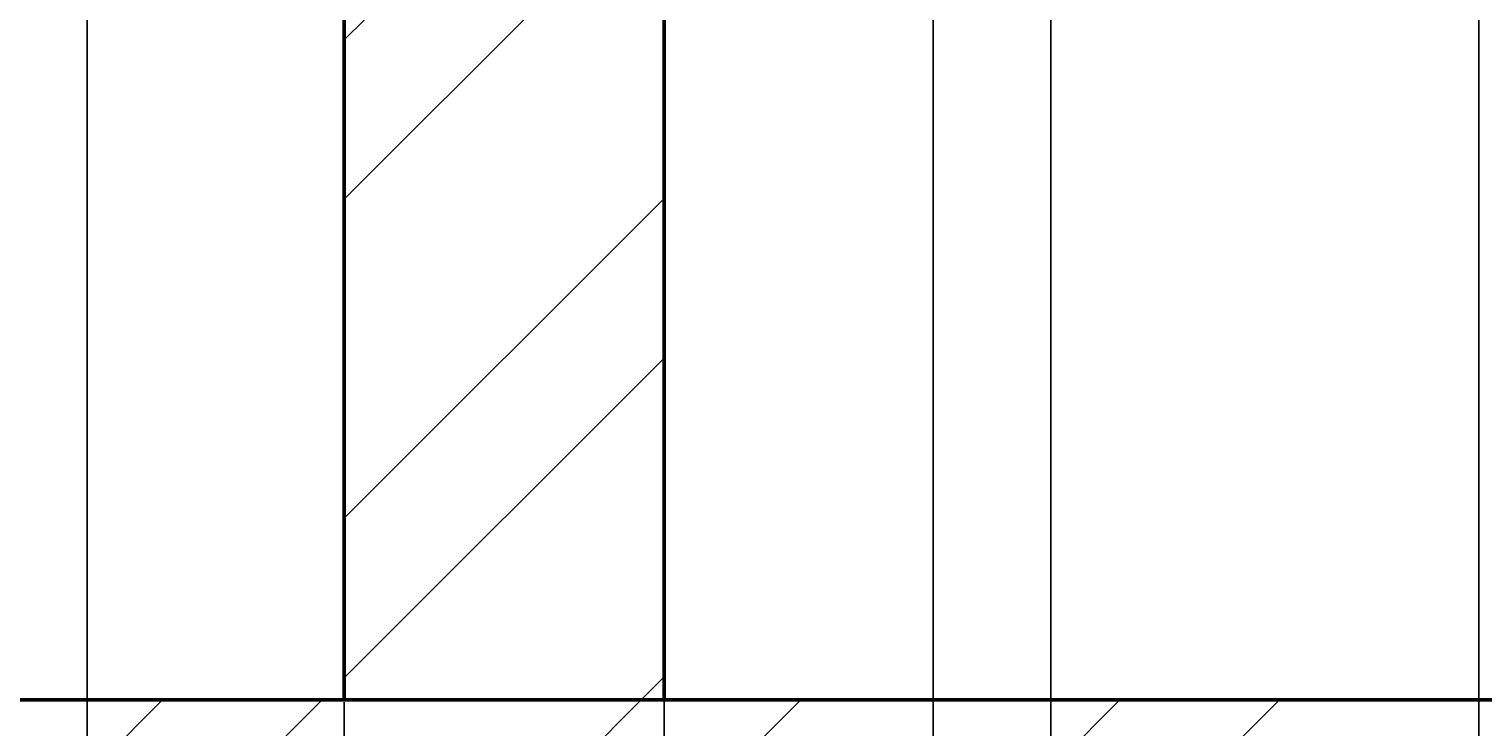
# Model space of a CAD drawing. Units: inches. Extents: x 2812 to 3051, y 1398 to 1659.
# Tile 58 of 65: x 2944 to 2984, y 1559 to 1579. Entities that reach past the tile are written whole.
import ezdxf

# ---------------------------------------------------------------- set-up
doc = ezdxf.new("R2010")
doc.units = ezdxf.units.IN
for name, color, linetype, lineweight in [('A-ANNO-DIMS', 2, 'Continuous', 18), ('S-CONC', 7, 'Continuous', 50), ('S-CONC-PATT', 8, 'Continuous', 18)]:
    doc.layers.add(name, color=color, linetype=linetype, lineweight=lineweight)
doc.styles.get("Standard").update_dxf_attribs({"font": 'arial.ttf'})
doc.dimstyles.get("Standard").update_dxf_attribs({"dimtxt": 0.18, "dimasz": 0.18, "dimexe": 0.18, "dimexo": 0.0625, "dimgap": 0.09, "dimtad": 0, "dimtih": 1, "dimtoh": 1, "dimdec": 4, "dimzin": 0, "dimdsep": 46, "dimtxsty": 'Standard', "dimcen": 0.09, "dimadec": 0, "dimazin": 0, "dimtfac": 1, "dimtdec": 4, "dimtofl": 0, "dimtmove": 0, "dimatfit": 3, "dimfxl": 1, "dimtolj": 1, "dimtzin": 0, "dimarcsym": 0})

# ---------------------------------------------------------------- blocks, each defined once
blk = doc.blocks.new('*D30')
at = {"layer": 'A-ANNO-DIMS', "color": 0, "lineweight": -2, "transparency": 16777216}
for p, q in [((2945.147, 1598.692), (2945.147, 1397.505)), ((2952.385, 1559.757), (2952.385, 1397.505)), ((2945.327, 1397.685), (2948.373, 1397.685)), ((2952.205, 1397.685), (2949.159, 1397.685))]:
    blk.add_line(p, q, dxfattribs=at)
at = {"layer": 'A-ANNO-DIMS', "color": 0, "transparency": 16777216}
for points in [[(2945.327, 1397.715), (2945.327, 1397.655), (2945.147, 1397.685)], [(2952.205, 1397.715), (2952.205, 1397.655), (2952.385, 1397.685)]]:
    blk.add_solid(points, dxfattribs=at)
at = {"layer": 'Defpoints', "color": 0, "transparency": 16777216}
for p in [(2945.147, 1598.754), (2952.385, 1559.82), (2952.385, 1397.685)]:
    blk.add_point(p, dxfattribs=at)
at = {"layer": 'A-ANNO-DIMS', "color": 0, "transparency": 16777216, "insert": (2948.766, 1397.685), "char_height": 0.18, "attachment_point": 5}
blk.add_mtext('\\A1;7.238', dxfattribs=at)
blk = doc.blocks.new('*D31')
at = {"layer": 'A-ANNO-DIMS', "color": 0, "lineweight": -2, "transparency": 16777216}
for p, q in [((2972.272, 1594.192), (2972.272, 1397.505)), ((2961.385, 1559.757), (2961.385, 1397.505)), ((2961.565, 1397.685), (2966.373, 1397.685)), ((2972.092, 1397.685), (2967.283, 1397.685))]:
    blk.add_line(p, q, dxfattribs=at)
at = {"layer": 'A-ANNO-DIMS', "color": 0, "transparency": 16777216}
for points in [[(2961.565, 1397.715), (2961.565, 1397.655), (2961.385, 1397.685)], [(2972.092, 1397.715), (2972.092, 1397.655), (2972.272, 1397.685)]]:
    blk.add_solid(points, dxfattribs=at)
at = {"layer": 'Defpoints', "color": 0, "transparency": 16777216}
for p in [(2972.272, 1594.254), (2961.385, 1559.82), (2972.272, 1397.685)]:
    blk.add_point(p, dxfattribs=at)
at = {"layer": 'A-ANNO-DIMS', "color": 0, "transparency": 16777216, "insert": (2966.828, 1397.685), "char_height": 0.18, "attachment_point": 5}
blk.add_mtext('\\A1;10.887', dxfattribs=at)
blk = doc.blocks.new('*D32')
at = {"layer": 'A-ANNO-DIMS', "color": 0, "lineweight": -2, "transparency": 16777216}
for p, q in [((2984.316, 1598.757), (2984.316, 1397.505)), ((2972.272, 1594.192), (2972.272, 1397.505)), ((2972.452, 1397.685), (2977.839, 1397.685)), ((2984.136, 1397.685), (2978.748, 1397.685))]:
    blk.add_line(p, q, dxfattribs=at)
at = {"layer": 'A-ANNO-DIMS', "color": 0, "transparency": 16777216}
for points in [[(2972.452, 1397.715), (2972.452, 1397.655), (2972.272, 1397.685)], [(2984.136, 1397.715), (2984.136, 1397.655), (2984.316, 1397.685)]]:
    blk.add_solid(points, dxfattribs=at)
at = {"layer": 'Defpoints', "color": 0, "transparency": 16777216}
for p in [(2984.316, 1598.82), (2972.272, 1594.254), (2984.316, 1397.685)]:
    blk.add_point(p, dxfattribs=at)
at = {"layer": 'A-ANNO-DIMS', "color": 0, "transparency": 16777216, "insert": (2978.294, 1397.685), "char_height": 0.18, "attachment_point": 5}
blk.add_mtext('\\A1;12.044', dxfattribs=at)
blk = doc.blocks.new('*D69')
at = {"layer": 'A-ANNO-DIMS', "color": 0, "lineweight": -2, "transparency": 16777216}
for p, q in [((2961.385, 1472.098), (2961.385, 1659.35)), ((2961.565, 1659.17), (2964.795, 1659.17)), ((2968.776, 1659.17), (2965.546, 1659.17)), ((2968.956, 1467.81), (2968.956, 1659.35))]:
    blk.add_line(p, q, dxfattribs=at)
at = {"layer": 'A-ANNO-DIMS', "color": 0, "transparency": 16777216}
for points in [[(2961.565, 1659.2), (2961.565, 1659.14), (2961.385, 1659.17)], [(2968.776, 1659.2), (2968.776, 1659.14), (2968.956, 1659.17)]]:
    blk.add_solid(points, dxfattribs=at)
at = {"layer": 'Defpoints', "color": 0, "transparency": 16777216}
for p in [(2968.956, 1659.17), (2961.385, 1472.035), (2968.956, 1467.747)]:
    blk.add_point(p, dxfattribs=at)
at = {"layer": 'A-ANNO-DIMS', "color": 0, "transparency": 16777216, "insert": (2965.17, 1659.17), "char_height": 0.18, "attachment_point": 5}
blk.add_mtext('\\A1;7.571', dxfattribs=at)

msp = doc.modelspace()

# ---------------------------------------------------------------- hatches: boundary and pattern name
at = {"layer": 'S-CONC-PATT'}
h = msp.add_hatch(dxfattribs=at)
h.set_pattern_fill('ANSI32', color=256)
h.paths.add_polyline_path([(3027.3849, 1646.82), (2835.3849, 1646.82), (2835.3849, 1603.2296), (2844.3849, 1603.2296), (2844.3849, 1637.82), (3018.3849, 1637.82), (3018.3849, 1602.5441), (3027.3849, 1602.5441)])
h.paths.add_polyline_path([(2844.3849, 1594.2296), (2835.3849, 1594.2296), (2835.3849, 1550.82), (3027.3849, 1550.82), (3027.3849, 1593.5441), (3018.3849, 1593.5441), (3018.3849, 1559.82), (2844.3849, 1559.82)])
h.paths.add_polyline_path([(2844.3849, 1482.0354), (2835.3849, 1482.0354), (2835.3849, 1463.4959), (2844.3849, 1463.4959)])
h.paths.add_polyline_path([(2844.3849, 1461.4959), (2835.3849, 1461.4959), (2835.3849, 1416.0354), (2844.3849, 1416.0354)])
h.paths.add_polyline_path([(3027.3849, 1482.0354), (3018.3849, 1482.0354), (3018.3849, 1463.2854), (3027.3849, 1463.2854)])
h.paths.add_polyline_path([(3027.3849, 1461.2854), (3018.3849, 1461.2854), (3018.3849, 1416.0354), (3027.3849, 1416.0354)])
h.paths.add_polyline_path([(2961.3849, 1448.4738), (2952.3849, 1448.4738), (2952.3849, 1416.0354), (2961.3849, 1416.0354)])
h.paths.add_polyline_path([(2961.3849, 1462.3026), (2952.3849, 1462.3026), (2952.3849, 1450.4738), (2961.3849, 1450.4738)])
h.paths.add_polyline_path([(2961.3849, 1472.0354), (2952.3849, 1472.0354), (2952.3849, 1462.3026), (2961.3849, 1462.3026)])
h = msp.add_hatch(dxfattribs=at)
h.set_pattern_fill('ANSI32', color=256)
h.paths.add_polyline_path([(2961.3849, 1637.82), (2952.3849, 1637.82), (2952.3849, 1603.2541), (2961.3849, 1603.2541)])
h.paths.add_polyline_path([(2961.3849, 1594.2541), (2952.3849, 1594.2541), (2952.3849, 1559.82), (2961.3849, 1559.82)])
h.paths.add_polyline_path([(2883.3849, 1637.82), (2880.3849, 1637.82), (2880.3849, 1559.82), (2883.3849, 1559.82)])

# ---------------------------------------------------------------- linework, layer by layer
at = {"layer": 'S-CONC'}
for p, q in [((2952.3849, 1637.82), (2952.3849, 1559.82)), ((2961.3849, 1559.82), (2961.3849, 1637.82)), ((2844.3849, 1559.82), (3018.3849, 1559.82))]:
    msp.add_line(p, q, dxfattribs=at)

# ---------------------------------------------------------------- dimensions: what is measured, and where the dimension line sits
at = {"layer": 'A-ANNO-DIMS'}
for base, p1, p2, picture, middle in [((2968.9558, 1659.17), (2961.3849, 1472.0354), (2968.9558, 1467.7474), '*D69', (2965.1704, 1659.17)), ((2952.3849, 1397.6854), (2945.1467, 1598.7541), (2952.3849, 1559.82), '*D30', (2948.7658, 1397.6854)), ((2984.3156, 1397.6854), (2972.2716, 1594.2541), (2984.3156, 1598.82), '*D32', (2978.2936, 1397.6854)), ((2972.2716, 1397.6854), (2961.3849, 1559.82), (2972.2716, 1594.2541), '*D31', (2966.8282, 1397.6854))]:
    dim = msp.add_linear_dim(base=base, p1=p1, p2=p2, dimstyle='Standard', override={"dimdec": 3, "dimlfac": 1, "dimrnd": 0, "dimzin": 0, "dimdsep": 46, "dimlunit": 2}, dxfattribs=at)
    dim.commit()
    dim.dimension.update_dxf_attribs({"geometry": picture, "text_midpoint": middle})

doc.saveas('drawing.dxf')
